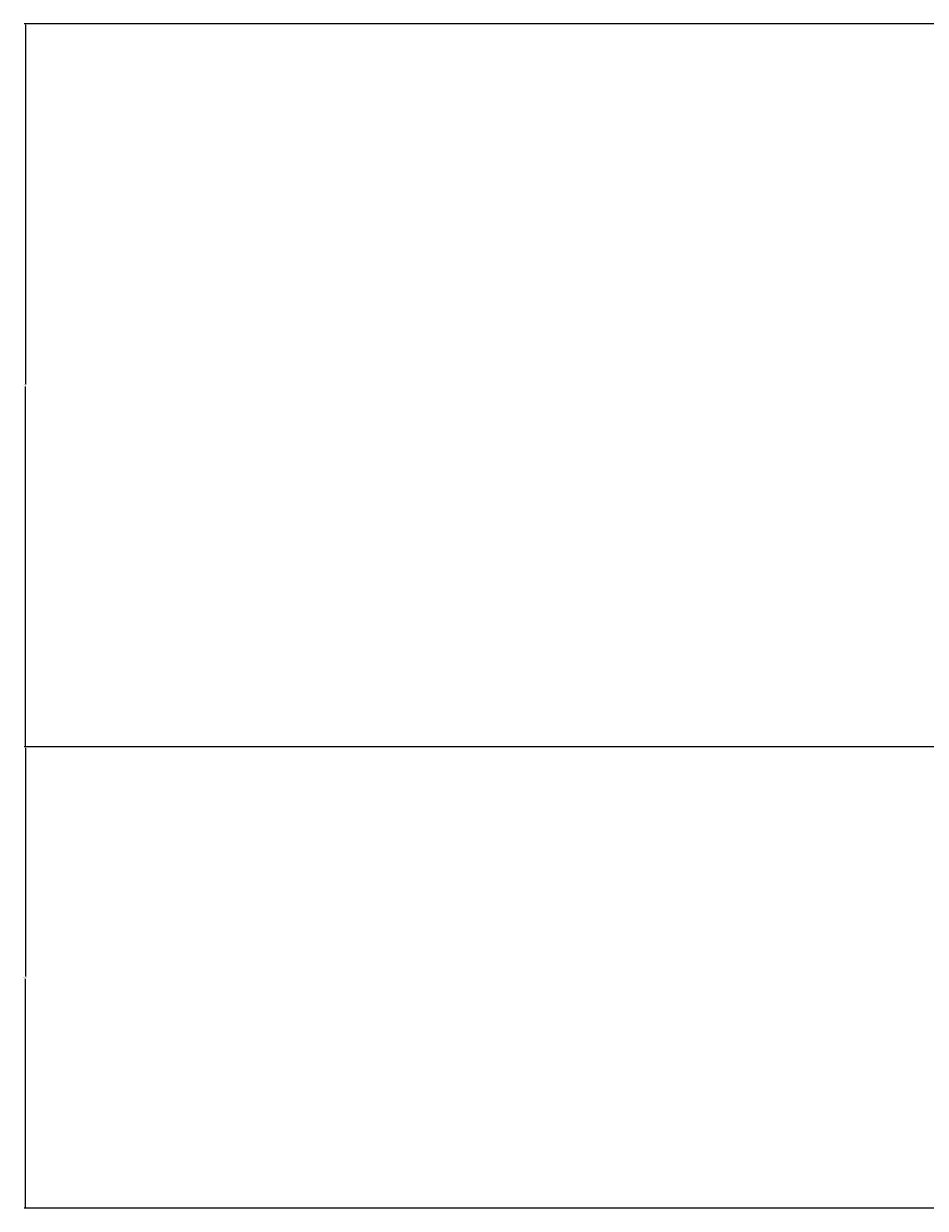
# Model space of a CAD drawing. Units: inches. Extents: x 338 to 1188, y -996 to 127.
# Tile 3 of 15: x 338 to 478, y -316 to -131. Entities that reach past the tile are written whole.
import ezdxf

# ---------------------------------------------------------------- set-up
doc = ezdxf.new("R2010")
doc.units = ezdxf.units.IN
doc.header["$MEASUREMENT"] = 0
doc.layers.add('A-ANNO-DIMS', color=5, linetype='Continuous', lineweight=18)
doc.styles.get("Standard").update_dxf_attribs({"font": 'arial.ttf'})
doc.dimstyles.get("Standard").update_dxf_attribs({"dimtxt": 0.18, "dimasz": 0.18, "dimexe": 0.18, "dimexo": 0.0625, "dimgap": 0.09, "dimtad": 0, "dimtih": 1, "dimtoh": 1, "dimdec": 1, "dimzin": 0, "dimdsep": 46, "dimlunit": 4, "dimtxsty": 'Standard', "dimcen": 0.09, "dimadec": 0, "dimazin": 0, "dimtfac": 1, "dimtdec": 1, "dimtofl": 0, "dimtmove": 0, "dimatfit": 3, "dimfxl": 1, "dimtolj": 1, "dimtzin": 0, "dimarcsym": 0})

# ---------------------------------------------------------------- blocks, each defined once
blk = doc.blocks.new('*D40')
at = {"layer": 'A-ANNO-DIMS', "color": 0, "lineweight": -2, "transparency": 16777216}
for p, q in [((596.9, -243.73), (337.66, -243.73)), ((337.84, -243.91), (337.84, -279.55)), ((337.84, -315.55), (337.84, -279.91)), ((596.9, -315.73), (337.66, -315.73))]:
    blk.add_line(p, q, dxfattribs=at)
at = {"layer": 'A-ANNO-DIMS', "color": 0, "transparency": 16777216}
for points in [[(337.81, -243.91), (337.87, -243.91), (337.84, -243.73)], [(337.81, -315.55), (337.87, -315.55), (337.84, -315.73)]]:
    blk.add_solid(points, dxfattribs=at)
at = {"layer": 'Defpoints', "color": 0, "transparency": 16777216}
for p in [(596.96, -243.73), (337.84, -315.73), (596.96, -315.73)]:
    blk.add_point(p, dxfattribs=at)
at = {"layer": 'A-ANNO-DIMS', "color": 0, "transparency": 16777216, "insert": (337.84, -279.73), "char_height": 0.18, "attachment_point": 5}
blk.add_mtext('\\A1;6\'-0"', dxfattribs=at)
blk = doc.blocks.new('*D51')
at = {"layer": 'A-ANNO-DIMS', "color": 0, "lineweight": -2, "transparency": 16777216}
for p, q in [((596.9, -130.89), (337.66, -130.89)), ((337.84, -131.07), (337.84, -187.13)), ((337.84, -243.55), (337.84, -187.49)), ((596.9, -243.73), (337.66, -243.73))]:
    blk.add_line(p, q, dxfattribs=at)
at = {"layer": 'A-ANNO-DIMS', "color": 0, "transparency": 16777216}
for points in [[(337.81, -131.07), (337.87, -131.07), (337.84, -130.89)], [(337.81, -243.55), (337.87, -243.55), (337.84, -243.73)]]:
    blk.add_solid(points, dxfattribs=at)
at = {"layer": 'Defpoints', "color": 0, "transparency": 16777216}
for p in [(596.96, -130.89), (337.84, -243.73), (596.96, -243.73)]:
    blk.add_point(p, dxfattribs=at)
at = {"layer": 'A-ANNO-DIMS', "color": 0, "transparency": 16777216, "insert": (337.84, -187.31), "char_height": 0.18, "attachment_point": 5}
blk.add_mtext('\\A1;9\'-5"', dxfattribs=at)

msp = doc.modelspace()

# ---------------------------------------------------------------- dimensions: what is measured, and where the dimension line sits
at = {"layer": 'A-ANNO-DIMS'}
for base, p1, p2, picture, middle in [((337.84, -243.73), (596.96, -130.89), (596.96, -243.73), '*D51', (337.84, -187.31)), ((337.84, -315.73), (596.96, -243.73), (596.96, -315.73), '*D40', (337.84, -279.73))]:
    dim = msp.add_linear_dim(base=base, p1=p1, p2=p2, angle=90, dimstyle='Standard', override={"dimdec": 1, "dimlfac": 1, "dimrnd": 0, "dimzin": 1, "dimdsep": 46, "dimlunit": 4, "dimfrac": 2}, dxfattribs=at)
    dim.commit()
    dim.dimension.update_dxf_attribs({"geometry": picture, "text_midpoint": middle})

doc.saveas('drawing.dxf')
